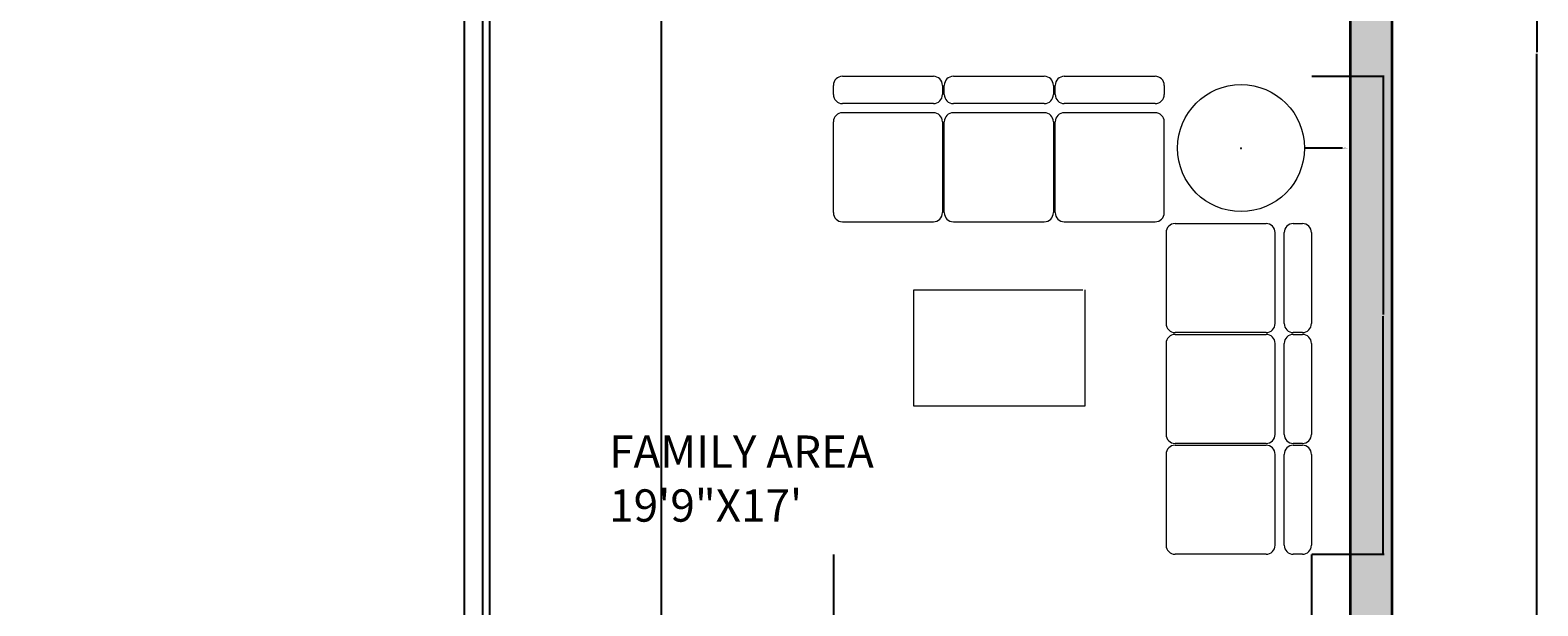
# Model space of a CAD drawing. Units: inches. Extents: x 1919 to 2461, y 2470 to 3159.
# Tile 5 of 6: x 2134 to 2461, y 2803 to 2928. Entities that reach past the tile are written whole.
import ezdxf

# ---------------------------------------------------------------- set-up
doc = ezdxf.new("R2010")
doc.units = ezdxf.units.IN
for name, color, linetype, lineweight in [('A-ANNO-DIMS', 2, 'Continuous', 18), ('A-AREA-IDEN', 7, 'Continuous', 18), ('A-FURN', 8, 'Continuous', 18), ('A-WALL', 7, 'Continuous', 35), ('A-WALL-PATT', 252, 'Continuous', 13)]:
    doc.layers.add(name, color=color, linetype=linetype, lineweight=lineweight)
doc.styles.get("Standard").update_dxf_attribs({"font": 'arial.ttf'})
doc.dimstyles.get("Standard").update_dxf_attribs({"dimtxt": 0.18, "dimasz": 0.18, "dimexe": 0.18, "dimexo": 0.0625, "dimgap": 0.09, "dimtad": 0, "dimtih": 1, "dimtoh": 1, "dimdec": 4, "dimzin": 0, "dimdsep": 46, "dimtxsty": 'Standard', "dimcen": 0.09, "dimadec": 0, "dimazin": 0, "dimtfac": 1, "dimtdec": 4, "dimtofl": 0, "dimtmove": 0, "dimatfit": 3, "dimfxl": 1, "dimtolj": 1, "dimtzin": 0, "dimarcsym": 0})

# ---------------------------------------------------------------- blocks, each defined once
blk = doc.blocks.new('A$C753D6792')
at = {"linetype": 'ByBlock'}
for p, q in [((0, 2530), (0, 2580)), ((50, 2630), (550, 2630)), ((600, 2580), (600, 2530)), ((610, 2530), (610, 2580)), ((660, 2630), (1160, 2630)), ((1210, 2580), (1210, 2530)), ((1220, 2530), (1220, 2580)), ((1270, 2630), (1770, 2630)), ((1820, 2580), (1820, 2530)), ((550, 2480), (50, 2480)), ((550, 2430), (50, 2430)), ((1160, 2480), (660, 2480)), ((1160, 2430), (660, 2430)), ((1770, 2480), (1270, 2480)), ((1770, 2430), (1270, 2430)), ((0, 1880), (0, 2380)), ((600, 2380), (600, 1880)), ((610, 1880), (610, 2380)), ((1210, 2380), (1210, 1880)), ((1220, 1880), (1220, 2380)), ((1820, 1880), (1820, 2380)), ((50, 1830), (427.2, 1830)), ((386.5, 1830), (550, 1830)), ((660, 1830), (1037.2, 1830)), ((996.5, 1830), (1160, 1830)), ((1270, 1830), (1647.2, 1830)), ((1606.5, 1830), (1770, 1830)), ((1830, 1770), (1830, 1392.8)), ((1880, 1820), (2380, 1820)), ((2430, 1270), (2430, 1770)), ((2480, 1270), (2480, 1770)), ((2530, 1820), (2580, 1820)), ((2630, 1770), (2630, 1270)), ((442.3, 815), (442.3, 1455)), ((442.3, 1455), (1372.3, 1455)), ((1382.3, 1455), (1382.3, 815)), ((1830, 1433.5), (1830, 1270)), ((2380, 1220), (1880, 1220)), ((1880, 1210), (2380, 1210)), ((2580, 1220), (2530, 1220)), ((2530, 1210), (2580, 1210)), ((1830, 1160), (1830, 782.8)), ((2430, 660), (2430, 1160)), ((2480, 660), (2480, 1160)), ((2630, 1160), (2630, 660)), ((1382.3, 815), (442.3, 815)), ((1830, 823.5), (1830, 660)), ((2380, 610), (1880, 610)), ((1880, 600), (2380, 600)), ((2580, 610), (2530, 610)), ((2530, 600), (2580, 600)), ((1830, 550), (1830, 172.8)), ((2430, 50), (2430, 550)), ((2480, 50), (2480, 550)), ((2630, 550), (2630, 50)), ((1830, 213.5), (1830, 50)), ((2380, 0), (1880, 0)), ((2580, 0), (2530, 0))]:
    blk.add_line(p, q, dxfattribs=at)
blk.add_circle((2242.3, 2235), 349.3, dxfattribs=at)
for centre, start, end in [((50, 2580), 90, 180), ((550, 2580), 0, 90), ((550, 2580), 0, 90), ((660, 2580), 90, 180), ((1160, 2580), 0, 90), ((1160, 2580), 0, 90), ((1270, 2580), 90, 180), ((1770, 2580), 0, 90), ((1770, 2580), 0, 90), ((50, 2530), 180, 270), ((550, 2530), 270, 0), ((550, 2530), 270, 0), ((660, 2530), 180, 270), ((1160, 2530), 270, 0), ((1160, 2530), 270, 0), ((1270, 2530), 180, 270), ((1770, 2530), 270, 0), ((1770, 2530), 270, 0), ((50, 2380), 90, 180), ((550, 2380), 0, 90), ((550, 2380), 0, 90), ((660, 2380), 90, 180), ((1160, 2380), 0, 90), ((1160, 2380), 0, 90), ((1270, 2380), 90, 180), ((1770, 2380), 0, 90), ((1770, 2380), 0, 90), ((50, 1880), 180, 270), ((550, 1880), 270, 0), ((660, 1880), 180, 270), ((1160, 1880), 270, 0), ((1270, 1880), 180, 270), ((1770, 1880), 270, 0), ((1880, 1770), 90, 180), ((2380, 1770), 0, 90), ((2530, 1770), 90, 180), ((2580, 1770), 0, 90), ((1880, 1270), 180, 270), ((2380, 1270), 270, 0), ((2380, 1270), 270, 0), ((2530, 1270), 180, 270), ((2530, 1270), 180, 270), ((2580, 1270), 270, 0), ((2580, 1270), 270, 0), ((1880, 1160), 90, 180), ((2380, 1160), 0, 90), ((2530, 1160), 90, 180), ((2580, 1160), 0, 90), ((1880, 660), 180, 270), ((1880, 550), 90, 180), ((2380, 660), 270, 0), ((2380, 660), 270, 0), ((2380, 550), 0, 90), ((2530, 660), 180, 270), ((2530, 660), 180, 270), ((2530, 550), 90, 180), ((2580, 660), 270, 0), ((2580, 660), 270, 0), ((2580, 550), 0, 90), ((1880, 50), 180, 270), ((2380, 50), 270, 0), ((2380, 50), 270, 0), ((2530, 50), 180, 270), ((2530, 50), 180, 270), ((2580, 50), 270, 0), ((2580, 50), 270, 0)]:
    blk.add_arc(centre, 50, start, end, dxfattribs=at)
blk = doc.blocks.new('*D11')
at = {"layer": 'A-ANNO-DIMS', "color": 0, "lineweight": -2, "transparency": 16777216}
for p, q in [((2308.31, 2814.5), (2308.31, 2798.86)), ((2411.85, 2814.5), (2411.85, 2798.86)), ((2308.49, 2799.04), (2358.71, 2799.04)), ((2411.67, 2799.04), (2361.45, 2799.04))]:
    blk.add_line(p, q, dxfattribs=at)
at = {"layer": 'A-ANNO-DIMS', "color": 0, "transparency": 16777216}
for points in [[(2308.49, 2799.07), (2308.49, 2799.01), (2308.31, 2799.04)], [(2411.67, 2799.07), (2411.67, 2799.01), (2411.85, 2799.04)]]:
    blk.add_solid(points, dxfattribs=at)
at = {"layer": 'Defpoints', "color": 0, "transparency": 16777216}
for p in [(2308.31, 2814.57), (2411.85, 2814.57), (2411.85, 2799.04)]:
    blk.add_point(p, dxfattribs=at)
at = {"layer": 'A-ANNO-DIMS', "color": 0, "transparency": 16777216, "insert": (2360.08, 2799.04), "char_height": 0.18, "attachment_point": 5}
blk.add_mtext('\\A1;SEATING GROUP 104', dxfattribs=at)
blk = doc.blocks.new('*D12')
at = {"layer": 'A-ANNO-DIMS', "color": 0, "lineweight": -2, "transparency": 16777216}
for p, q in [((2411.92, 2918.11), (2427.57, 2918.11)), ((2427.39, 2917.93), (2427.39, 2866.52)), ((2427.39, 2814.75), (2427.39, 2866.16)), ((2411.92, 2814.57), (2427.57, 2814.57))]:
    blk.add_line(p, q, dxfattribs=at)
at = {"layer": 'A-ANNO-DIMS', "color": 0, "transparency": 16777216}
for points in [[(2427.36, 2917.93), (2427.42, 2917.93), (2427.39, 2918.11)], [(2427.36, 2814.75), (2427.42, 2814.75), (2427.39, 2814.57)]]:
    blk.add_solid(points, dxfattribs=at)
at = {"layer": 'Defpoints', "color": 0, "transparency": 16777216}
for p in [(2411.85, 2918.11), (2427.39, 2918.11), (2411.85, 2814.57)]:
    blk.add_point(p, dxfattribs=at)
at = {"layer": 'A-ANNO-DIMS', "color": 0, "transparency": 16777216, "insert": (2427.39, 2866.34), "char_height": 0.18, "attachment_point": 5}
blk.add_mtext('\\A1;104', dxfattribs=at)
blk = doc.blocks.new('*D36')
at = {"layer": 'A-ANNO-DIMS', "color": 0, "lineweight": -2, "transparency": 16777216}
for p, q in [((2429.38, 3127.67), (2460.85, 3127.67)), ((2460.67, 3127.49), (2460.67, 2923.35)), ((2460.67, 2718.85), (2460.67, 2922.99)), ((2429.38, 2718.67), (2460.85, 2718.67))]:
    blk.add_line(p, q, dxfattribs=at)
at = {"layer": 'A-ANNO-DIMS', "color": 0, "transparency": 16777216}
for points in [[(2460.64, 3127.49), (2460.7, 3127.49), (2460.67, 3127.67)], [(2460.64, 2718.85), (2460.7, 2718.85), (2460.67, 2718.67)]]:
    blk.add_solid(points, dxfattribs=at)
at = {"layer": 'Defpoints', "color": 0, "transparency": 16777216}
for p in [(2429.32, 3127.67), (2460.67, 3127.67), (2429.32, 2718.67)]:
    blk.add_point(p, dxfattribs=at)
at = {"layer": 'A-ANNO-DIMS', "color": 0, "transparency": 16777216, "insert": (2460.67, 2923.17), "char_height": 0.18, "attachment_point": 5}
blk.add_mtext('\\A1;409', dxfattribs=at)
blk = doc.blocks.new('*D42')
at = {"layer": 'A-ANNO-DIMS', "color": 0, "lineweight": -2, "transparency": 16777216}
for p, q in [((2233.88, 2630.46), (2233.88, 3159.21)), ((2234.06, 3159.03), (2252.1, 3159.03)), ((2270.93, 3159.03), (2252.89, 3159.03)), ((2271.11, 2661.64), (2271.11, 3159.21))]:
    blk.add_line(p, q, dxfattribs=at)
at = {"layer": 'A-ANNO-DIMS', "color": 0, "transparency": 16777216}
for points in [[(2234.06, 3159.06), (2234.06, 3159), (2233.88, 3159.03)], [(2270.93, 3159.06), (2270.93, 3159), (2271.11, 3159.03)]]:
    blk.add_solid(points, dxfattribs=at)
at = {"layer": 'Defpoints', "color": 0, "transparency": 16777216}
for p in [(2271.11, 3159.03), (2271.11, 2661.57), (2233.88, 2630.39)]:
    blk.add_point(p, dxfattribs=at)
at = {"layer": 'A-ANNO-DIMS', "color": 0, "transparency": 16777216, "insert": (2252.49, 3159.03), "char_height": 0.18, "attachment_point": 5}
blk.add_mtext('\\A1;37.23', dxfattribs=at)
blk = doc.blocks.new('*D43')
at = {"layer": 'A-ANNO-DIMS', "color": 0, "lineweight": -2, "transparency": 16777216}
for p, q in [((2228.32, 2940.61), (2228.32, 2470.14)), ((2232.32, 2940.61), (2232.32, 2470.14)), ((2228.5, 2470.32), (2230.16, 2470.32)), ((2232.14, 2470.32), (2230.47, 2470.32))]:
    blk.add_line(p, q, dxfattribs=at)
at = {"layer": 'A-ANNO-DIMS', "color": 0, "transparency": 16777216}
for points in [[(2228.5, 2470.35), (2228.5, 2470.29), (2228.32, 2470.32)], [(2232.14, 2470.35), (2232.14, 2470.29), (2232.32, 2470.32)]]:
    blk.add_solid(points, dxfattribs=at)
at = {"layer": 'Defpoints', "color": 0, "transparency": 16777216}
for p in [(2228.32, 2940.67), (2232.32, 2940.67), (2232.32, 2470.32)]:
    blk.add_point(p, dxfattribs=at)
at = {"layer": 'A-ANNO-DIMS', "color": 0, "transparency": 16777216, "insert": (2230.32, 2470.32), "char_height": 0.18, "attachment_point": 5}
blk.add_mtext('\\A1;4', dxfattribs=at)
blk = doc.blocks.new('*D51')
at = {"layer": 'A-ANNO-DIMS', "color": 0, "lineweight": -2, "transparency": 16777216}
for p, q in [((2396.5, 2902.56), (2396.68, 2902.56)), ((2396.59, 2902.47), (2396.59, 2902.65)), ((2418.59, 2902.56), (2410.52, 2902.56))]:
    blk.add_line(p, q, dxfattribs=at)
at = {"layer": 'A-ANNO-DIMS', "color": 0, "transparency": 16777216}
blk.add_solid([(2410.52, 2902.59), (2410.52, 2902.53), (2410.34, 2902.56)], dxfattribs=at)
at = {"layer": 'Defpoints', "color": 0, "transparency": 16777216}
for p in [(2382.84, 2902.56), (2410.34, 2902.56)]:
    blk.add_point(p, dxfattribs=at)
at = {"layer": 'A-ANNO-DIMS', "color": 0, "transparency": 16777216, "insert": (2419.16, 2902.56), "char_height": 0.18, "attachment_point": 5}
blk.add_mtext('\\A1;∅27.503', dxfattribs=at)

msp = doc.modelspace()

# ---------------------------------------------------------------- hatches: boundary and pattern name
at = {"layer": 'A-WALL-PATT'}
h = msp.add_hatch(color=256, dxfattribs=at)
h.dxf.hatch_style = 1
h.paths.add_polyline_path([(1959.315, 2931.672), (2066.315, 2931.672), (2066.315, 2940.672), (2062.315, 2940.672), (2062.315, 3005.672), (2066.315, 3005.672), (2066.315, 3009.672), (2062.315, 3009.672), (2062.315, 3118.672), (2062.315, 3127.672), (2004.315, 3127.672), (2004.315, 3072.672), (1950.315, 3072.672), (1950.315, 3059.672), (1959.315, 3059.672), (1959.315, 3063.672), (2017.315, 3063.672), (2017.315, 3067.672), (2013.315, 3067.672), (2013.315, 3118.672), (2058.315, 3118.672), (2058.315, 3067.672), (2047.315, 3067.672), (2047.315, 3063.672), (2058.315, 3063.672), (2058.315, 2940.672), (1959.315, 2940.672), (1959.315, 2952.172), (1950.315, 2952.172), (1950.315, 2901.672), (1959.315, 2901.672)])
h.paths.add_polyline_path([(2120.315, 2791.672), (2145.315, 2791.672), (2145.315, 2795.672), (2124.315, 2795.672), (2124.315, 2803.3999), (2115.315, 2803.3999), (2115.315, 2799.3999), (2067.5871, 2751.672), (1959.315, 2751.672), (1959.315, 2781.672), (1950.315, 2781.672), (1950.315, 2718.672), (1959.315, 2718.672), (1959.315, 2742.672), (2067.315, 2742.672), (2067.315, 2670.672), (2063.315, 2670.672), (2063.315, 2666.672), (2143.3108, 2666.672, 0.09553844), (2136.315, 2630.3938), (2145.315, 2630.3938, -0.2455558), (2183.315, 2703.1037), (2183.315, 2713.8315, 0.15123975), (2145.0175, 2670.672), (2071.315, 2670.672), (2071.315, 2742.672)])
h.paths.add_polyline_path([(2124.315, 2931.672), (2232.315, 2931.672), (2232.315, 2940.672), (2228.315, 2940.672), (2228.315, 2964.672), (2219.315, 2964.672), (2219.315, 2940.672), (2138.315, 2940.672), (2138.315, 3005.672), (2185.315, 3005.672), (2185.315, 3009.672), (2138.315, 3009.672), (2138.315, 3118.672), (2138.315, 3127.672), (2086.315, 3127.672), (2086.315, 3118.672), (2134.315, 3118.672), (2134.315, 3009.672), (2096.315, 3009.672), (2096.315, 3005.672), (2134.315, 3005.672), (2134.315, 2940.672), (2096.315, 2940.672), (2096.315, 2931.672), (2115.315, 2931.672), (2115.315, 2839.3999), (2124.315, 2839.3999)])
h.paths.add_polyline_path([(2429.315, 3127.672), (2384.315, 3127.672), (2384.315, 3118.672), (2420.315, 3118.672), (2420.315, 2940.672), (2268.315, 2940.672), (2268.315, 2931.672), (2420.315, 2931.672), (2420.315, 2727.672), (2364.3064, 2727.672), (2317.4188, 2680.7844, 0.0404216), (2308.2227, 2693.5694), (2301.7735, 2687.2567, -0.63673951), (2233.8773, 2541.8315), (2145.315, 2541.8315), (2145.315, 2594.3938), (2136.315, 2594.3938), (2136.315, 2510.672), (2107.815, 2510.672), (2107.815, 2501.672), (2145.315, 2501.672), (2145.315, 2532.8315), (2233.8773, 2532.8315, 0.55190633), (2321.8781, 2672.5158), (2368.0343, 2718.672), (2429.315, 2718.672)])
h.paths.add_polyline_path([(2228.315, 3118.672), (2264.315, 3118.672), (2264.315, 3127.672), (2162.315, 3127.672), (2162.315, 3118.672), (2219.315, 3118.672), (2219.315, 3009.672), (2215.315, 3009.672), (2215.315, 3005.672), (2219.315, 3005.672), (2219.315, 2994.672), (2228.315, 2994.672)], flags=0)
h.paths.add_polyline_path([(1959.315, 2666.672), (2033.315, 2666.672), (2033.315, 2670.672), (1959.315, 2670.672), (1959.315, 2694.672), (1950.315, 2694.672), (1950.315, 2501.672), (1987.815, 2501.672), (1987.815, 2510.672), (1959.315, 2510.672)])

# ---------------------------------------------------------------- linework, layer by layer
at = {"layer": 'A-WALL'}
for p, q in [((2429.315, 2718.672), (2429.315, 3127.672)), ((2420.315, 2727.672), (2420.315, 2931.672))]:
    msp.add_line(p, q, dxfattribs=at)

# ---------------------------------------------------------------- block references
at = {"layer": 'A-FURN', "xscale": 0.0393700787401575, "yscale": 0.0393700787401575, "zscale": 0.0393700787401575}
msp.add_blockref('A$C753D6792', (2308.3105, 2814.5671), dxfattribs=at)

# ---------------------------------------------------------------- texts
at = {"layer": 'A-AREA-IDEN', "insert": (2259.7478, 2840.3038), "char_height": 7, "attachment_point": 1}
msp.add_mtext_dynamic_manual_height_columns('FAMILY AREA\\P19\'9"X17\'', width=121.344683, gutter_width=12.5, heights=[0], dxfattribs=at)

# ---------------------------------------------------------------- dimensions: what is measured, and where the dimension line sits
at = {"layer": 'A-ANNO-DIMS'}
for base, p1, p2, override, picture, middle in [((2271.1076, 3159.027), (2233.8773, 2630.3938), (2271.1076, 2661.574), {"dimdec": 2, "dimlfac": 1, "dimrnd": 0, "dimzin": 0, "dimdsep": 46, "dimlunit": 2}, '*D42', (2252.4924, 3159.027)), ((2232.315, 2470.317), (2228.315, 2940.672), (2232.315, 2940.672), {"dimdec": 0, "dimlfac": 1, "dimrnd": 0, "dimzin": 0, "dimdsep": 46, "dimlunit": 2}, '*D43', (2230.315, 2470.317))]:
    dim = msp.add_linear_dim(base=base, p1=p1, p2=p2, dimstyle='Standard', override=override, dxfattribs=at)
    dim.commit()
    dim.dimension.update_dxf_attribs({"geometry": picture, "text_midpoint": middle})
for base, p1, p2, picture, middle in [((2460.67, 3127.672), (2429.315, 2718.672), (2429.315, 3127.672), '*D36', (2460.67, 2923.172)), ((2427.3853, 2918.1104), (2411.8538, 2814.5671), (2411.8538, 2918.1104), '*D12', (2427.3853, 2866.3387))]:
    dim = msp.add_linear_dim(base=base, p1=p1, p2=p2, angle=90, dimstyle='Standard', override={"dimdec": 0, "dimlfac": 1, "dimrnd": 0, "dimzin": 0, "dimdsep": 46, "dimlunit": 2}, dxfattribs=at)
    dim.commit()
    dim.dimension.update_dxf_attribs({"geometry": picture, "text_midpoint": middle})
dim = msp.add_diameter_dim_2p(p1=(2382.8399, 2902.5594), p2=(2410.3427, 2902.559), dimstyle='Standard', override={"dimdec": 3, "dimlfac": 1, "dimrnd": 0, "dimzin": 0, "dimdsep": 46, "dimlunit": 2}, dxfattribs=at)
dim.commit()
dim.dimension.update_dxf_attribs({"geometry": '*D51', "text_midpoint": (2418.5935, 2902.5589), "dimtype": 163})
dim = msp.add_linear_dim(base=(2411.8538, 2799.0356), p1=(2308.3105, 2814.5671), p2=(2411.8538, 2814.5671), text='SEATING GROUP <>', dimstyle='Standard', override={"dimdec": 0, "dimlfac": 1, "dimrnd": 0, "dimzin": 0, "dimdsep": 46, "dimlunit": 2}, dxfattribs=at)
dim.commit()
dim.dimension.update_dxf_attribs({"geometry": '*D11', "text_midpoint": (2360.0821, 2799.0356)})

doc.saveas('drawing.dxf')
